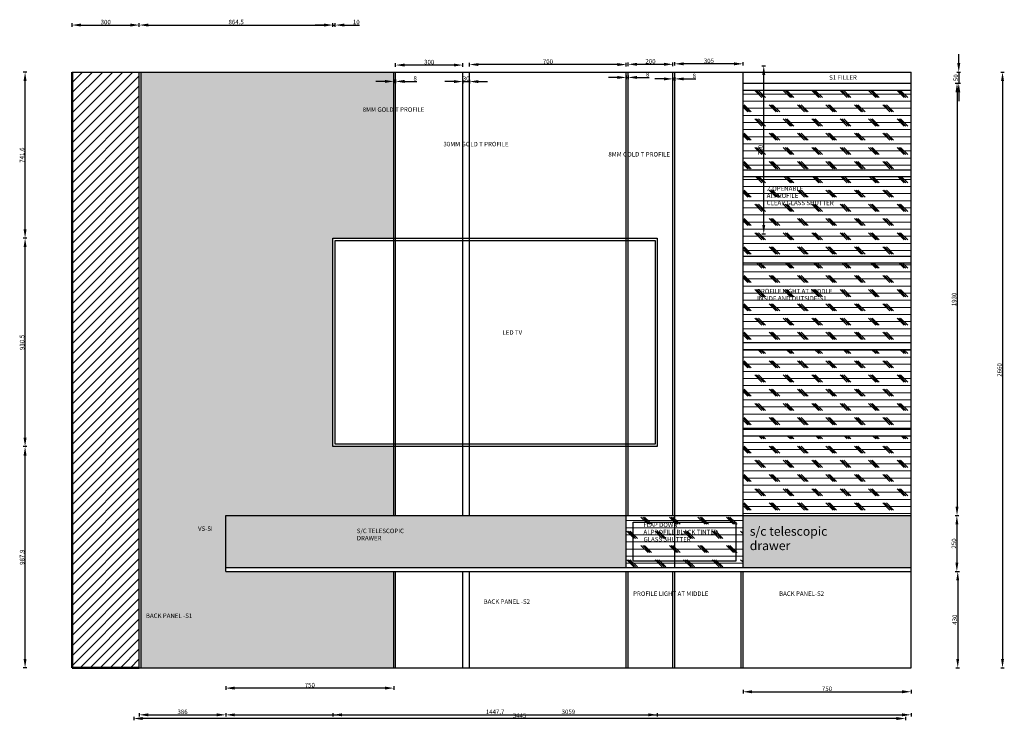
# Model space of a CAD drawing. Units: millimetres. Extents: x -4231 to 8464, y -424 to 4269.
# Tile 2 of 2: x 4069 to 8464, y 1141 to 4269. Entities that reach past the tile are written whole.
import ezdxf

# ---------------------------------------------------------------- set-up
doc = ezdxf.new("R2010")
doc.units = ezdxf.units.MM
for name, color, linetype, lineweight in [('A-ANNO-DIMS', 2, 'Continuous', 18), ('A-ANNO-TEXT', 3, 'Continuous', 18), ('A-EQPM', 6, 'Continuous', 25), ('A-FURN', 30, 'Continuous', 25), ('A-FURN-PATT', 252, 'Continuous', 13), ('A-WALL', 7, 'Continuous', 50), ('A-WALL-PATT', 8, 'Continuous', 13)]:
    doc.layers.add(name, color=color, linetype=linetype, lineweight=lineweight)
doc.styles.get("Standard").update_dxf_attribs({"font": 'arial.ttf', "height": 20})
doc.dimstyles.new('ISO-25', dxfattribs={"dimtxt": 40, "dimasz": 40, "dimexe": 8, "dimexo": 8, "dimtad": 1, "dimdec": 0, "dimtxsty": 'Standard', "dimcen": 2.5, "dimadec": 0, "dimazin": 0, "dimtfac": 1, "dimtdec": 0, "dimtmove": 0, "dimatfit": 3, "dimfxl": 8, "dimfxlon": 1, "dimarcsym": 0})
pattern_1 = [(0, (0, 0), (0, 31.75), []), (135, (15.875, -15.875), (-63.5, -63.5), [44.9013, -44.9013]), (135, (23.81, -15.875), (-63.5, -63.5), [44.9013, -44.9013]), (135, (31.75, -15.875), (-63.5, -63.5), [44.9013, -44.9013])]

# ---------------------------------------------------------------- blocks, each defined once
blk = doc.blocks.new('*D14')
at = {"layer": 'A-ANNO-DIMS', "color": 0, "lineweight": -2, "transparency": 16777216}
for p, q in [((7382.1, 4062.6), (7398.1, 4062.6)), ((7390.1, 3352.6), (7390.1, 4022.6)), ((7382.1, 3312.6), (7398.1, 3312.6))]:
    blk.add_line(p, q, dxfattribs=at)
at = {"layer": 'A-ANNO-DIMS', "color": 0, "transparency": 16777216}
for points in [[(7383.5, 4022.6), (7396.8, 4022.6), (7390.1, 4062.6)], [(7383.5, 3352.6), (7396.8, 3352.6), (7390.1, 3312.6)]]:
    blk.add_solid(points, dxfattribs=at)
at = {"layer": 'Defpoints', "color": 0, "transparency": 16777216}
for p in [(7351.4, 4062.6), (7390.1, 4062.6), (7351.4, 3312.6)]:
    blk.add_point(p, dxfattribs=at)
at = {"layer": 'A-ANNO-DIMS', "color": 0, "transparency": 16777216, "insert": (7379.3, 3687.6), "char_height": 20, "attachment_point": 5, "rotation": 90}
blk.add_mtext('750', dxfattribs=at)
blk = doc.blocks.new('*D15')
at = {"layer": 'A-ANNO-DIMS', "color": 0, "lineweight": -2, "transparency": 16777216}
for p, q in [((6784.7, 4061.8), (6784.7, 4077.8)), ((6824.7, 4069.8), (6944.7, 4069.8)), ((6984.7, 4061.8), (6984.7, 4077.8))]:
    blk.add_line(p, q, dxfattribs=at)
at = {"layer": 'A-ANNO-DIMS', "color": 0, "transparency": 16777216}
for points in [[(6824.7, 4076.5), (6824.7, 4063.2), (6784.7, 4069.8)], [(6944.7, 4076.5), (6944.7, 4063.2), (6984.7, 4069.8)]]:
    blk.add_solid(points, dxfattribs=at)
at = {"layer": 'Defpoints', "color": 0, "transparency": 16777216}
for p in [(6984.7, 4069.8), (6784.7, 4035), (6984.7, 4035)]:
    blk.add_point(p, dxfattribs=at)
at = {"layer": 'A-ANNO-DIMS', "color": 0, "transparency": 16777216, "insert": (6884.7, 4080.7), "char_height": 20, "attachment_point": 5}
blk.add_mtext('200', dxfattribs=at)
blk = doc.blocks.new('*D16')
at = {"layer": 'A-ANNO-DIMS', "color": 0, "lineweight": -2, "transparency": 16777216}
for p, q in [((6992.7, 4063.8), (6992.7, 4079.8)), ((7257.7, 4071.8), (7032.7, 4071.8)), ((7297.7, 4063.8), (7297.7, 4079.8))]:
    blk.add_line(p, q, dxfattribs=at)
at = {"layer": 'A-ANNO-DIMS', "color": 0, "transparency": 16777216}
for points in [[(7032.7, 4078.5), (7032.7, 4065.1), (6992.7, 4071.8)], [(7257.7, 4078.5), (7257.7, 4065.1), (7297.7, 4071.8)]]:
    blk.add_solid(points, dxfattribs=at)
at = {"layer": 'Defpoints', "color": 0, "transparency": 16777216}
for p in [(6992.7, 4071.8), (6992.7, 4035), (7297.7, 4035)]:
    blk.add_point(p, dxfattribs=at)
at = {"layer": 'A-ANNO-DIMS', "color": 0, "transparency": 16777216, "insert": (7145.2, 4082.7), "char_height": 20, "attachment_point": 5}
blk.add_mtext('305', dxfattribs=at)
blk = doc.blocks.new('*D17')
at = {"layer": 'A-ANNO-DIMS', "color": 0, "lineweight": -2, "transparency": 16777216}
for p, q in [((6076.7, 4060.7), (6076.7, 4076.7)), ((6736.7, 4068.7), (6116.7, 4068.7)), ((6776.7, 4060.7), (6776.7, 4076.7))]:
    blk.add_line(p, q, dxfattribs=at)
at = {"layer": 'A-ANNO-DIMS', "color": 0, "transparency": 16777216}
for points in [[(6116.7, 4075.3), (6116.7, 4062), (6076.7, 4068.7)], [(6736.7, 4075.3), (6736.7, 4062), (6776.7, 4068.7)]]:
    blk.add_solid(points, dxfattribs=at)
at = {"layer": 'Defpoints', "color": 0, "transparency": 16777216}
for p in [(6076.7, 4068.7), (6076.7, 4035), (6776.7, 4035)]:
    blk.add_point(p, dxfattribs=at)
at = {"layer": 'A-ANNO-DIMS', "color": 0, "transparency": 16777216, "insert": (6426.7, 4079.5), "char_height": 20, "attachment_point": 5}
blk.add_mtext('700', dxfattribs=at)
blk = doc.blocks.new('*D18')
at = {"layer": 'A-ANNO-DIMS', "color": 0, "lineweight": -2, "transparency": 16777216}
for p, q in [((5746.7, 4058.4), (5746.7, 4074.4)), ((6006.7, 4066.4), (5786.7, 4066.4)), ((6046.7, 4058.4), (6046.7, 4074.4))]:
    blk.add_line(p, q, dxfattribs=at)
at = {"layer": 'A-ANNO-DIMS', "color": 0, "transparency": 16777216}
for points in [[(5786.7, 4073.1), (5786.7, 4059.8), (5746.7, 4066.4)], [(6006.7, 4073.1), (6006.7, 4059.8), (6046.7, 4066.4)]]:
    blk.add_solid(points, dxfattribs=at)
at = {"layer": 'Defpoints', "color": 0, "transparency": 16777216}
for p in [(5746.7, 4066.4), (5746.7, 4035), (6046.7, 4035)]:
    blk.add_point(p, dxfattribs=at)
at = {"layer": 'A-ANNO-DIMS', "color": 0, "transparency": 16777216, "insert": (5896.7, 4077.3), "char_height": 20, "attachment_point": 5}
blk.add_mtext('300', dxfattribs=at)
blk = doc.blocks.new('*D19')
at = {"layer": 'A-ANNO-DIMS', "color": 0, "lineweight": -2, "transparency": 16777216}
for p, q in [((8260.7, 4075), (8260.7, 4115)), ((8252.7, 4035), (8268.7, 4035)), ((8260.7, 4035), (8260.7, 3985)), ((8252.7, 3985), (8268.7, 3985)), ((8260.7, 3945), (8260.7, 3905))]:
    blk.add_line(p, q, dxfattribs=at)
at = {"layer": 'A-ANNO-DIMS', "color": 0, "transparency": 16777216}
for points in [[(8254, 4075), (8267.3, 4075), (8260.7, 4035)], [(8254, 3945), (8267.3, 3945), (8260.7, 3985)]]:
    blk.add_solid(points, dxfattribs=at)
at = {"layer": 'Defpoints', "color": 0, "transparency": 16777216}
for p in [(8047.7, 4035), (8047.7, 3985), (8260.7, 3985)]:
    blk.add_point(p, dxfattribs=at)
at = {"layer": 'A-ANNO-DIMS', "color": 0, "transparency": 16777216, "insert": (8249.8, 4010), "char_height": 20, "attachment_point": 5, "rotation": 90}
blk.add_mtext('50', dxfattribs=at)
blk = doc.blocks.new('*D20')
at = {"layer": 'A-ANNO-DIMS', "color": 0, "lineweight": -2, "transparency": 16777216}
for p, q in [((8245, 3985), (8261, 3985)), ((8253, 3945), (8253, 2095)), ((8245, 2055), (8261, 2055))]:
    blk.add_line(p, q, dxfattribs=at)
at = {"layer": 'A-ANNO-DIMS', "color": 0, "transparency": 16777216}
for points in [[(8246.3, 3945), (8259.6, 3945), (8253, 3985)], [(8246.3, 2095), (8259.6, 2095), (8253, 2055)]]:
    blk.add_solid(points, dxfattribs=at)
at = {"layer": 'Defpoints', "color": 0, "transparency": 16777216}
for p in [(8047.7, 3985), (8047.7, 2055), (8253, 2055)]:
    blk.add_point(p, dxfattribs=at)
at = {"layer": 'A-ANNO-DIMS', "color": 0, "transparency": 16777216, "insert": (8242.1, 3020), "char_height": 20, "attachment_point": 5, "rotation": 90}
blk.add_mtext('1930', dxfattribs=at)
blk = doc.blocks.new('*D21')
at = {"layer": 'A-ANNO-DIMS', "color": 0, "lineweight": -2, "transparency": 16777216}
for p, q in [((8448, 4035), (8464, 4035)), ((8456, 3995), (8456, 1415)), ((8448, 1375), (8464, 1375))]:
    blk.add_line(p, q, dxfattribs=at)
at = {"layer": 'A-ANNO-DIMS', "color": 0, "transparency": 16777216}
for points in [[(8449.4, 3995), (8462.7, 3995), (8456, 4035)], [(8449.4, 1415), (8462.7, 1415), (8456, 1375)]]:
    blk.add_solid(points, dxfattribs=at)
at = {"layer": 'Defpoints', "color": 0, "transparency": 16777216}
for p in [(8047.7, 4035), (8047.7, 1375), (8456, 1375)]:
    blk.add_point(p, dxfattribs=at)
at = {"layer": 'A-ANNO-DIMS', "color": 0, "transparency": 16777216, "insert": (8445.2, 2705), "char_height": 20, "attachment_point": 5, "rotation": 90}
blk.add_mtext('2660', dxfattribs=at)
blk = doc.blocks.new('*D22')
at = {"layer": 'A-ANNO-DIMS', "color": 0, "lineweight": -2, "transparency": 16777216}
for p, q in [((8248.1, 1805), (8264.1, 1805)), ((8256.1, 1765), (8256.1, 1415)), ((8248.1, 1375), (8264.1, 1375))]:
    blk.add_line(p, q, dxfattribs=at)
at = {"layer": 'A-ANNO-DIMS', "color": 0, "transparency": 16777216}
for points in [[(8249.4, 1765), (8262.7, 1765), (8256.1, 1805)], [(8249.4, 1415), (8262.7, 1415), (8256.1, 1375)]]:
    blk.add_solid(points, dxfattribs=at)
at = {"layer": 'Defpoints', "color": 0, "transparency": 16777216}
for p in [(8047.7, 1805), (8047.7, 1375), (8256.1, 1375)]:
    blk.add_point(p, dxfattribs=at)
at = {"layer": 'A-ANNO-DIMS', "color": 0, "transparency": 16777216, "insert": (8245.2, 1590), "char_height": 20, "attachment_point": 5, "rotation": 90}
blk.add_mtext('430', dxfattribs=at)
blk = doc.blocks.new('*D23')
at = {"layer": 'A-ANNO-DIMS', "color": 0, "lineweight": -2, "transparency": 16777216}
for p, q in [((8244.3, 2055), (8260.3, 2055)), ((8252.3, 2015), (8252.3, 1845)), ((8244.3, 1805), (8260.3, 1805))]:
    blk.add_line(p, q, dxfattribs=at)
at = {"layer": 'A-ANNO-DIMS', "color": 0, "transparency": 16777216}
for points in [[(8245.7, 2015), (8259, 2015), (8252.3, 2055)], [(8245.7, 1845), (8259, 1845), (8252.3, 1805)]]:
    blk.add_solid(points, dxfattribs=at)
at = {"layer": 'Defpoints', "color": 0, "transparency": 16777216}
for p in [(8047.7, 2055), (8047.7, 1805), (8252.3, 1805)]:
    blk.add_point(p, dxfattribs=at)
at = {"layer": 'A-ANNO-DIMS', "color": 0, "transparency": 16777216, "insert": (8241.5, 1930), "char_height": 20, "attachment_point": 5, "rotation": 90}
blk.add_mtext('250', dxfattribs=at)
blk = doc.blocks.new('*D24')
at = {"layer": 'A-ANNO-DIMS', "color": 0, "lineweight": -2, "transparency": 16777216}
for p, q in [((7297.7, 1276.1), (7297.7, 1260.1)), ((8047.7, 1276.1), (8047.7, 1260.1)), ((7337.7, 1268.1), (8007.7, 1268.1))]:
    blk.add_line(p, q, dxfattribs=at)
at = {"layer": 'A-ANNO-DIMS', "color": 0, "transparency": 16777216}
for points in [[(7337.7, 1274.8), (7337.7, 1261.4), (7297.7, 1268.1)], [(8007.7, 1274.8), (8007.7, 1261.4), (8047.7, 1268.1)]]:
    blk.add_solid(points, dxfattribs=at)
at = {"layer": 'Defpoints', "color": 0, "transparency": 16777216}
for p in [(7297.7, 1823), (8047.7, 1823), (8047.7, 1268.1)]:
    blk.add_point(p, dxfattribs=at)
at = {"layer": 'A-ANNO-DIMS', "color": 0, "transparency": 16777216, "insert": (7672.7, 1278.9), "char_height": 20, "attachment_point": 5}
blk.add_mtext('750', dxfattribs=at)
blk = doc.blocks.new('*D25')
at = {"layer": 'A-ANNO-DIMS', "color": 0, "lineweight": -2, "transparency": 16777216}
for p, q in [((4988.7, 1292.4), (4988.7, 1276.4)), ((5698.7, 1284.4), (5028.7, 1284.4)), ((5738.7, 1292.4), (5738.7, 1276.4))]:
    blk.add_line(p, q, dxfattribs=at)
at = {"layer": 'A-ANNO-DIMS', "color": 0, "transparency": 16777216}
for points in [[(5028.7, 1291.1), (5028.7, 1277.7), (4988.7, 1284.4)], [(5698.7, 1291.1), (5698.7, 1277.7), (5738.7, 1284.4)]]:
    blk.add_solid(points, dxfattribs=at)
at = {"layer": 'Defpoints', "color": 0, "transparency": 16777216}
for p in [(4988.7, 1375), (5738.7, 1375), (4988.7, 1284.4)]:
    blk.add_point(p, dxfattribs=at)
at = {"layer": 'A-ANNO-DIMS', "color": 0, "transparency": 16777216, "insert": (5363.7, 1295.2), "char_height": 20, "attachment_point": 5}
blk.add_mtext('750', dxfattribs=at)
blk = doc.blocks.new('*D26')
at = {"layer": 'A-ANNO-DIMS', "color": 0, "lineweight": -2, "transparency": 16777216}
for p, q in [((4577.6, 1156.6), (4577.6, 1140.6)), ((7982.6, 1148.6), (4617.6, 1148.6)), ((8022.6, 1156.6), (8022.6, 1140.6))]:
    blk.add_line(p, q, dxfattribs=at)
at = {"layer": 'A-ANNO-DIMS', "color": 0, "transparency": 16777216}
for points in [[(4617.6, 1155.3), (4617.6, 1141.9), (4577.6, 1148.6)], [(7982.6, 1155.3), (7982.6, 1141.9), (8022.6, 1148.6)]]:
    blk.add_solid(points, dxfattribs=at)
at = {"layer": 'Defpoints', "color": 0, "transparency": 16777216}
for p in [(4577.6, 1631.7), (8022.6, 1631.7), (4577.6, 1148.6)]:
    blk.add_point(p, dxfattribs=at)
at = {"layer": 'A-ANNO-DIMS', "color": 0, "transparency": 16777216, "insert": (6300.1, 1159.4), "char_height": 20, "attachment_point": 5}
blk.add_mtext('3445', dxfattribs=at)
blk = doc.blocks.new('*D27')
at = {"layer": 'A-ANNO-DIMS', "color": 0, "lineweight": -2, "transparency": 16777216}
for p, q in [((5738.7, 4001.3), (5738.7, 3985.3)), ((5746.7, 4001.3), (5746.7, 3985.3)), ((5698.7, 3993.3), (5658.7, 3993.3)), ((5738.7, 3993.3), (5746.7, 3993.3)), ((5786.7, 3993.3), (5841.1, 3993.3))]:
    blk.add_line(p, q, dxfattribs=at)
at = {"layer": 'A-ANNO-DIMS', "color": 0, "transparency": 16777216}
for points in [[(5698.7, 4000), (5698.7, 3986.6), (5738.7, 3993.3)], [(5786.7, 4000), (5786.7, 3986.6), (5746.7, 3993.3)]]:
    blk.add_solid(points, dxfattribs=at)
at = {"layer": 'Defpoints', "color": 0, "transparency": 16777216}
for p in [(5738.7, 4035), (5746.7, 4035), (5746.7, 3993.3)]:
    blk.add_point(p, dxfattribs=at)
at = {"layer": 'A-ANNO-DIMS', "color": 0, "transparency": 16777216, "insert": (5833.9, 4004.1), "char_height": 20, "attachment_point": 5}
blk.add_mtext('8', dxfattribs=at)
blk = doc.blocks.new('*D28')
at = {"layer": 'A-ANNO-DIMS', "color": 0, "lineweight": -2, "transparency": 16777216}
for p, q in [((6046.7, 4000.6), (6046.7, 3984.6)), ((6076.7, 4000.6), (6076.7, 3984.6)), ((6006.7, 3992.6), (5966.7, 3992.6)), ((6046.7, 3992.6), (6076.7, 3992.6)), ((6116.7, 3992.6), (6156.7, 3992.6))]:
    blk.add_line(p, q, dxfattribs=at)
at = {"layer": 'A-ANNO-DIMS', "color": 0, "transparency": 16777216}
for points in [[(6006.7, 3999.2), (6006.7, 3985.9), (6046.7, 3992.6)], [(6116.7, 3999.2), (6116.7, 3985.9), (6076.7, 3992.6)]]:
    blk.add_solid(points, dxfattribs=at)
at = {"layer": 'Defpoints', "color": 0, "transparency": 16777216}
for p in [(6046.7, 4035), (6076.7, 4035), (6076.7, 3992.6)]:
    blk.add_point(p, dxfattribs=at)
at = {"layer": 'A-ANNO-DIMS', "color": 0, "transparency": 16777216, "insert": (6061.7, 4003.4), "char_height": 20, "attachment_point": 5}
blk.add_mtext('30', dxfattribs=at)
blk = doc.blocks.new('*D29')
at = {"layer": 'A-ANNO-DIMS', "color": 0, "lineweight": -2, "transparency": 16777216}
for p, q in [((6736.7, 4011.1), (6696.7, 4011.1)), ((6776.7, 4019.1), (6776.7, 4003.1)), ((6776.7, 4011.1), (6784.7, 4011.1)), ((6784.7, 4019.1), (6784.7, 4003.1)), ((6824.7, 4011.1), (6879.1, 4011.1))]:
    blk.add_line(p, q, dxfattribs=at)
at = {"layer": 'A-ANNO-DIMS', "color": 0, "transparency": 16777216}
for points in [[(6736.7, 4017.8), (6736.7, 4004.5), (6776.7, 4011.1)], [(6824.7, 4017.8), (6824.7, 4004.5), (6784.7, 4011.1)]]:
    blk.add_solid(points, dxfattribs=at)
at = {"layer": 'Defpoints', "color": 0, "transparency": 16777216}
for p in [(6776.7, 4035), (6784.7, 4035), (6784.7, 4011.1)]:
    blk.add_point(p, dxfattribs=at)
at = {"layer": 'A-ANNO-DIMS', "color": 0, "transparency": 16777216, "insert": (6871.9, 4022), "char_height": 20, "attachment_point": 5}
blk.add_mtext('8', dxfattribs=at)
blk = doc.blocks.new('*D30')
at = {"layer": 'A-ANNO-DIMS', "color": 0, "lineweight": -2, "transparency": 16777216}
for p, q in [((6944.7, 4004.6), (6904.7, 4004.6)), ((6984.7, 4012.6), (6984.7, 3996.6)), ((6984.7, 4004.6), (6992.7, 4004.6)), ((6992.7, 4012.6), (6992.7, 3996.6)), ((7032.7, 4004.6), (7087.1, 4004.6))]:
    blk.add_line(p, q, dxfattribs=at)
at = {"layer": 'A-ANNO-DIMS', "color": 0, "transparency": 16777216}
for points in [[(6944.7, 4011.2), (6944.7, 3997.9), (6984.7, 4004.6)], [(7032.7, 4011.2), (7032.7, 3997.9), (6992.7, 4004.6)]]:
    blk.add_solid(points, dxfattribs=at)
at = {"layer": 'Defpoints', "color": 0, "transparency": 16777216}
for p in [(6984.7, 4035), (6992.7, 4035), (6992.7, 4004.6)]:
    blk.add_point(p, dxfattribs=at)
at = {"layer": 'A-ANNO-DIMS', "color": 0, "transparency": 16777216, "insert": (7079.9, 4015.4), "char_height": 20, "attachment_point": 5}
blk.add_mtext('8', dxfattribs=at)
blk = doc.blocks.new('*D34')
at = {"layer": 'A-ANNO-DIMS', "color": 0, "lineweight": -2, "transparency": 16777216}
for p, q in [((4302.7, 4237), (4302.7, 4253)), ((4342.7, 4245), (4562.7, 4245)), ((4602.7, 4237), (4602.7, 4253))]:
    blk.add_line(p, q, dxfattribs=at)
at = {"layer": 'A-ANNO-DIMS', "color": 0, "transparency": 16777216}
for points in [[(4342.7, 4251.7), (4342.7, 4238.4), (4302.7, 4245)], [(4562.7, 4251.7), (4562.7, 4238.4), (4602.7, 4245)]]:
    blk.add_solid(points, dxfattribs=at)
at = {"layer": 'Defpoints', "color": 0, "transparency": 16777216}
for p in [(4602.7, 4245), (4302.7, 4035), (4602.7, 4035)]:
    blk.add_point(p, dxfattribs=at)
at = {"layer": 'A-ANNO-DIMS', "color": 0, "transparency": 16777216, "insert": (4452.7, 4255.9), "char_height": 20, "attachment_point": 5}
blk.add_mtext('300', dxfattribs=at)
blk = doc.blocks.new('*D35')
at = {"layer": 'A-ANNO-DIMS', "color": 0, "lineweight": -2, "transparency": 16777216}
for p, q in [((4602.7, 4237), (4602.7, 4253)), ((4642.7, 4245), (5427.2, 4245)), ((5467.2, 4237), (5467.2, 4253))]:
    blk.add_line(p, q, dxfattribs=at)
at = {"layer": 'A-ANNO-DIMS', "color": 0, "transparency": 16777216}
for points in [[(4642.7, 4251.7), (4642.7, 4238.4), (4602.7, 4245)], [(5427.2, 4251.7), (5427.2, 4238.4), (5467.2, 4245)]]:
    blk.add_solid(points, dxfattribs=at)
at = {"layer": 'Defpoints', "color": 0, "transparency": 16777216}
for p in [(5467.2, 4245), (4602.7, 4035), (5467.2, 3293.4)]:
    blk.add_point(p, dxfattribs=at)
at = {"layer": 'A-ANNO-DIMS', "color": 0, "transparency": 16777216, "insert": (5034.9, 4255.9), "char_height": 20, "attachment_point": 5}
blk.add_mtext('864.5', dxfattribs=at)
blk = doc.blocks.new('*D36')
at = {"layer": 'A-ANNO-DIMS', "color": 0, "lineweight": -2, "transparency": 16777216}
for p, q in [((5427.2, 4245), (5387.2, 4245)), ((5467.2, 4237), (5467.2, 4253)), ((5467.2, 4245), (5477.2, 4245)), ((5477.2, 4237), (5477.2, 4253)), ((5517.2, 4245), (5585.1, 4245))]:
    blk.add_line(p, q, dxfattribs=at)
at = {"layer": 'A-ANNO-DIMS', "color": 0, "transparency": 16777216}
for points in [[(5427.2, 4251.7), (5427.2, 4238.4), (5467.2, 4245)], [(5517.2, 4251.7), (5517.2, 4238.4), (5477.2, 4245)]]:
    blk.add_solid(points, dxfattribs=at)
at = {"layer": 'Defpoints', "color": 0, "transparency": 16777216}
for p in [(5477.2, 4245), (5467.2, 3293.4), (5477.2, 3283.4)]:
    blk.add_point(p, dxfattribs=at)
at = {"layer": 'A-ANNO-DIMS', "color": 0, "transparency": 16777216, "insert": (5571.2, 4255.9), "char_height": 20, "attachment_point": 5}
blk.add_mtext('10', dxfattribs=at)
blk = doc.blocks.new('*D37')
at = {"layer": 'A-ANNO-DIMS', "color": 0, "lineweight": -2, "transparency": 16777216}
for p, q in [((4602.7, 1173), (4602.7, 1157)), ((4642.7, 1165), (4948.7, 1165)), ((4988.7, 1173), (4988.7, 1157))]:
    blk.add_line(p, q, dxfattribs=at)
at = {"layer": 'A-ANNO-DIMS', "color": 0, "transparency": 16777216}
for points in [[(4642.7, 1171.7), (4642.7, 1158.4), (4602.7, 1165)], [(4948.7, 1171.7), (4948.7, 1158.4), (4988.7, 1165)]]:
    blk.add_solid(points, dxfattribs=at)
at = {"layer": 'Defpoints', "color": 0, "transparency": 16777216}
for p in [(4988.7, 1805), (4602.7, 1375), (4988.7, 1165)]:
    blk.add_point(p, dxfattribs=at)
at = {"layer": 'A-ANNO-DIMS', "color": 0, "transparency": 16777216, "insert": (4795.7, 1175.9), "char_height": 20, "attachment_point": 5}
blk.add_mtext('386', dxfattribs=at)
blk = doc.blocks.new('*D38')
at = {"layer": 'A-ANNO-DIMS', "color": 0, "lineweight": -2, "transparency": 16777216}
for p, q in [((4988.7, 1173), (4988.7, 1157)), ((5028.7, 1165), (8007.7, 1165)), ((8047.7, 1173), (8047.7, 1157))]:
    blk.add_line(p, q, dxfattribs=at)
at = {"layer": 'A-ANNO-DIMS', "color": 0, "transparency": 16777216}
for points in [[(5028.7, 1171.7), (5028.7, 1158.4), (4988.7, 1165)], [(8007.7, 1171.7), (8007.7, 1158.4), (8047.7, 1165)]]:
    blk.add_solid(points, dxfattribs=at)
at = {"layer": 'Defpoints', "color": 0, "transparency": 16777216}
for p in [(4988.7, 1805), (8047.7, 1375), (8047.7, 1165)]:
    blk.add_point(p, dxfattribs=at)
at = {"layer": 'A-ANNO-DIMS', "color": 0, "transparency": 16777216, "insert": (6518.2, 1175.9), "char_height": 20, "attachment_point": 5}
blk.add_mtext('3059', dxfattribs=at)
blk = doc.blocks.new('*D39')
at = {"layer": 'A-ANNO-DIMS', "color": 0, "lineweight": -2, "transparency": 16777216}
for p, q in [((5467.2, 1173), (5467.2, 1157)), ((5507.2, 1165), (6874.9, 1165)), ((6914.9, 1173), (6914.9, 1157))]:
    blk.add_line(p, q, dxfattribs=at)
at = {"layer": 'A-ANNO-DIMS', "color": 0, "transparency": 16777216}
for points in [[(5507.2, 1171.7), (5507.2, 1158.4), (5467.2, 1165)], [(6874.9, 1171.7), (6874.9, 1158.4), (6914.9, 1165)]]:
    blk.add_solid(points, dxfattribs=at)
at = {"layer": 'Defpoints', "color": 0, "transparency": 16777216}
for p in [(5467.2, 2362.9), (6914.9, 2362.9), (6914.9, 1165)]:
    blk.add_point(p, dxfattribs=at)
at = {"layer": 'A-ANNO-DIMS', "color": 0, "transparency": 16777216, "insert": (6191, 1175.7), "char_height": 20, "attachment_point": 5}
blk.add_mtext('1447.7', dxfattribs=at)
blk = doc.blocks.new('*D40')
at = {"layer": 'A-ANNO-DIMS', "color": 0, "lineweight": -2, "transparency": 16777216}
for p, q in [((4100.7, 2362.9), (4084.7, 2362.9)), ((4092.7, 1415), (4092.7, 2322.9)), ((4100.7, 1375), (4084.7, 1375))]:
    blk.add_line(p, q, dxfattribs=at)
at = {"layer": 'A-ANNO-DIMS', "color": 0, "transparency": 16777216}
for points in [[(4086, 2322.9), (4099.3, 2322.9), (4092.7, 2362.9)], [(4086, 1415), (4099.3, 1415), (4092.7, 1375)]]:
    blk.add_solid(points, dxfattribs=at)
at = {"layer": 'Defpoints', "color": 0, "transparency": 16777216}
for p in [(4092.7, 2362.9), (5467.2, 2362.9), (4302.7, 1375)]:
    blk.add_point(p, dxfattribs=at)
at = {"layer": 'A-ANNO-DIMS', "color": 0, "transparency": 16777216, "insert": (4081.8, 1869), "char_height": 20, "attachment_point": 5, "rotation": 90}
blk.add_mtext('987.9', dxfattribs=at)
blk = doc.blocks.new('*D41')
at = {"layer": 'A-ANNO-DIMS', "color": 0, "lineweight": -2, "transparency": 16777216}
for p, q in [((4100.7, 3293.4), (4084.7, 3293.4)), ((4092.7, 2402.9), (4092.7, 3253.4)), ((4100.7, 2362.9), (4084.7, 2362.9))]:
    blk.add_line(p, q, dxfattribs=at)
at = {"layer": 'A-ANNO-DIMS', "color": 0, "transparency": 16777216}
for points in [[(4086, 3253.4), (4099.3, 3253.4), (4092.7, 3293.4)], [(4086, 2402.9), (4099.3, 2402.9), (4092.7, 2362.9)]]:
    blk.add_solid(points, dxfattribs=at)
at = {"layer": 'Defpoints', "color": 0, "transparency": 16777216}
for p in [(4092.7, 3293.4), (5467.2, 3293.4), (5467.2, 2362.9)]:
    blk.add_point(p, dxfattribs=at)
at = {"layer": 'A-ANNO-DIMS', "color": 0, "transparency": 16777216, "insert": (4081.8, 2828.1), "char_height": 20, "attachment_point": 5, "rotation": 90}
blk.add_mtext('930.5', dxfattribs=at)
blk = doc.blocks.new('*D42')
at = {"layer": 'A-ANNO-DIMS', "color": 0, "lineweight": -2, "transparency": 16777216}
for p, q in [((4100.7, 4035), (4084.7, 4035)), ((4092.7, 3333.4), (4092.7, 3995)), ((4100.7, 3293.4), (4084.7, 3293.4))]:
    blk.add_line(p, q, dxfattribs=at)
at = {"layer": 'A-ANNO-DIMS', "color": 0, "transparency": 16777216}
for points in [[(4086, 3995), (4099.3, 3995), (4092.7, 4035)], [(4086, 3333.4), (4099.3, 3333.4), (4092.7, 3293.4)]]:
    blk.add_solid(points, dxfattribs=at)
at = {"layer": 'Defpoints', "color": 0, "transparency": 16777216}
for p in [(4092.7, 4035), (4302.7, 4035), (5467.2, 3293.4)]:
    blk.add_point(p, dxfattribs=at)
at = {"layer": 'A-ANNO-DIMS', "color": 0, "transparency": 16777216, "insert": (4081.8, 3664.2), "char_height": 20, "attachment_point": 5, "rotation": 90}
blk.add_mtext('741.6', dxfattribs=at)

msp = doc.modelspace()

# ---------------------------------------------------------------- hatches: boundary and pattern name
at = {"layer": 'A-FURN-PATT'}
h = msp.add_hatch(dxfattribs=at)
h.set_pattern_fill('GOST_WOOD', color=256, scale=10)
h.paths.add_polyline_path([(5738.65, 4035.02), (4610.65, 4035.02), (4610.65, 1375.02), (5738.65, 1375.02), (5738.65, 1805.02), (4988.65, 1805.02), (4988.65, 2055.02), (5738.65, 2055.02), (5738.65, 2362.91), (5467.19, 2362.91), (5467.19, 3293.39), (5738.65, 3293.39)])
h.paths.add_polyline_path([(6776.65, 2055.02), (4988.65, 2055.02), (4988.65, 1823.02), (6776.65, 1823.02)])
h.paths.add_polyline_path([(8047.65, 2055.02), (7297.65, 2055.02), (7297.65, 1823.02), (8047.65, 1823.02)])
h.paths.add_polyline_path([(4626.95, 1591.95), (4864, 1591.95), (4864, 1622.97), (4626.95, 1622.97)], flags=24)
h.paths.add_polyline_path([(4859.72, 1980.87), (4943.03, 1980.87), (4943.03, 2011.9), (4859.72, 2011.9)], flags=24)
h.paths.add_polyline_path([(5568.61, 1939.16), (5702.79, 1939.16), (5702.79, 1969.16), (5568.61, 1969.16)], flags=24)
h.paths.add_polyline_path([(5568.44, 1970.77), (5810.12, 1970.77), (5810.12, 2001.81), (5568.44, 2001.81)], flags=24)
h.paths.add_polyline_path([(7317.55, 1889.74), (7509.45, 1889.74), (7509.45, 1950.72), (7317.55, 1950.72)], flags=24)
h.paths.add_polyline_path([(7314.77, 1940.76), (7691.61, 1940.76), (7691.61, 2018.44), (7314.77, 2018.44)], flags=24)
h = msp.add_hatch(dxfattribs=at)
h.set_pattern_fill('CORK', color=256, scale=10)
h.set_pattern_definition(pattern_1)
h.paths.add_polyline_path([(8047.65, 3955.02), (7297.65, 3955.02), (7297.65, 3599.02), (8047.65, 3599.02)])
h.paths.add_polyline_path([(8047.65, 3569.02), (7297.65, 3569.02), (7297.65, 3213.02), (8047.65, 3213.02)])
h.paths.add_polyline_path([(8047.65, 3183.02), (7297.65, 3183.02), (7297.65, 2827.02), (8047.65, 2827.02)])
h.paths.add_polyline_path([(8047.65, 2797.02), (7297.65, 2797.02), (7297.65, 2441.02), (8047.65, 2441.02)])
h.paths.add_polyline_path([(8047.65, 2411.02), (7297.65, 2411.02), (7297.65, 2055.02), (8047.65, 2055.02)])
h = msp.add_hatch(dxfattribs=at)
h.set_pattern_fill('CORK', color=256, scale=10)
h.set_pattern_definition(pattern_1)
h.paths.add_polyline_path([(7267.65, 2025.02), (6992.65, 2025.02), (6806.65, 2025.02), (6806.65, 1853.02), (7267.65, 1853.02)], flags=0)
h.paths.add_polyline_path([(7297.65, 2055.02), (6992.65, 2055.02), (6776.65, 2055.02), (6776.65, 1823.02), (7297.65, 1823.02)])
h.paths.add_polyline_path([(7267.65, 1853.02), (6806.65, 1853.02), (6806.65, 2025.02), (6992.65, 2025.02), (7267.65, 2025.02)], flags=16)
h = msp.add_hatch(dxfattribs=at)
h.set_pattern_fill('CORK', color=256, scale=10)
h.set_pattern_definition(pattern_1)
h.paths.add_polyline_path([(7267.65, 2025.02), (6992.65, 2025.02), (6806.65, 2025.02), (6806.65, 1853.02), (7267.65, 1853.02)])
at = {"layer": 'A-WALL-PATT'}
h = msp.add_hatch(dxfattribs=at)
h.set_pattern_fill('ANSI31', color=256, scale=10)
h.paths.add_polyline_path([(4602.65, 4035.02), (4302.65, 4035.02), (4302.65, 1375.02), (4602.65, 1375.02)])

# ---------------------------------------------------------------- linework, layer by layer
at = {"layer": 'A-EQPM'}
for points in [[(5467.19, 3293.39), (6914.85, 3293.39), (6914.85, 2362.91), (5467.19, 2362.91)], [(5477.19, 3283.39), (6904.85, 3283.39), (6904.85, 2372.91), (5477.19, 2372.91)]]:
    msp.add_lwpolyline(points, close=True, dxfattribs=at)
at = {"layer": 'A-FURN'}
for p, q in [((4302.65, 4035.02), (8047.65, 4035.02)), ((4602.65, 1375.02), (4602.65, 4035.02)), ((4610.65, 1375.02), (4610.65, 4035.02)), ((5738.65, 2055.02), (5738.65, 4035.02)), ((5746.65, 2055.02), (5746.65, 4035.02)), ((6046.65, 2055.02), (6046.65, 4035.02)), ((6076.65, 2055.02), (6076.65, 4035.02)), ((6776.65, 1823.02), (6776.65, 4035.02)), ((6784.65, 2055.02), (6784.65, 4035.02)), ((6984.65, 2055.02), (6984.65, 4035.02)), ((6992.65, 2055.02), (6992.65, 4035.02)), ((6992.65, 1823.02), (6992.65, 4035.02)), ((6992.65, 1823.02), (6992.65, 4035.02)), ((6992.65, 1823.02), (6992.65, 4035.02)), ((7297.65, 1823.02), (7297.65, 4035.02)), ((8047.65, 1375.02), (8047.65, 4035.02)), ((7297.65, 3985.02), (8047.65, 3985.02)), ((7297.65, 3955.02), (8047.65, 3955.02)), ((7297.65, 3599.02), (8047.65, 3599.02)), ((7297.65, 3569.02), (8047.65, 3569.02)), ((7297.65, 3213.02), (8047.65, 3213.02)), ((7297.65, 3183.02), (8047.65, 3183.02)), ((7297.65, 2827.02), (8047.65, 2827.02)), ((7297.65, 2797.02), (8047.65, 2797.02)), ((7297.65, 2441.02), (8047.65, 2441.02)), ((7297.65, 2411.02), (8047.65, 2411.02)), ((4988.65, 2055.02), (6992.65, 2055.02)), ((4988.65, 1805.02), (4988.65, 2055.02)), ((6806.65, 2025.02), (6992.65, 2025.02)), ((6806.65, 1853.02), (6806.65, 2025.02)), ((6992.65, 2055.02), (8047.65, 2055.02)), ((6992.65, 2025.02), (7267.65, 2025.02)), ((7267.65, 1853.02), (7267.65, 2025.02)), ((6806.65, 1853.02), (7267.65, 1853.02)), ((4988.65, 1823.02), (8047.65, 1823.02)), ((4988.65, 1805.02), (8047.65, 1805.02)), ((5738.65, 1375.02), (5738.65, 1805.02)), ((5746.65, 1375.02), (5746.65, 1805.02)), ((6046.65, 1375.02), (6046.65, 1805.02)), ((6076.65, 1375.02), (6076.65, 1805.02)), ((6776.65, 1375.02), (6776.65, 1805.02)), ((6784.65, 1375.02), (6784.65, 1805.02)), ((6984.65, 1375.02), (6984.65, 1805.02)), ((6992.65, 1375.02), (6992.65, 1805.02)), ((7289.65, 1375.02), (7289.65, 1805.02)), ((7297.65, 1375.02), (7297.65, 1805.02)), ((4602.65, 1375.02), (8047.65, 1375.02))]:
    msp.add_line(p, q, dxfattribs=at)
at = {"layer": 'A-WALL'}
for p, q in [((4302.65, 1375.02), (4302.65, 4035.02)), ((4602.65, 1375.02), (4302.65, 1375.02))]:
    msp.add_line(p, q, dxfattribs=at)

# ---------------------------------------------------------------- texts
at = {"layer": 'A-ANNO-TEXT'}
for s, height, p in [('S1 FILLER', 20, (7682.18, 4000.52)), ('8MM GOLD T PROFILE', 20, (5600.02, 3857.57)), ('30MM GOLD T PROFILE', 20, (5960.27, 3703.56)), ('8MM GOLD T PROFILE', 20, (6696.51, 3657.91)), ('2-OPENABLE', 20, (7403.33, 3505.02)), ('AI.PROFILE', 20, (7403.33, 3472.9)), ('CLEAR GLASS SHUTTER', 20, (7403.33, 3440.77)), ('PROFILE LIGHT AT MIDDLE', 20, (7360.25, 3047.11)), ('INSIDE AND OUTSIDE-S1', 20, (7360.25, 3014.98)), ('LED TV', 20, (6223.87, 2862.49)), ('FLAP DOWN', 20, (6853.39, 2003.25)), ('VS-SI', 20, (4864.89, 1986.39)), ('S/C TELESCOPIC', 20, (5573.61, 1976.28)), ('AI.PROFILE BLACK TINTED', 20, (6853.39, 1971.12)), ('s/c telescopic ', 40, (7327.72, 1964.81)), ('DRAWER', 20, (5573.61, 1944.16)), ('GLASS SHUTTER', 20, (6853.39, 1938.99)), ('drawer', 40, (7327.72, 1900.56)), ('PROFILE LIGHT AT MIDDLE  ', 20, (6806.87, 1695.92)), ('BACK PANEL-S2', 20, (7458.48, 1696.22)), ('BACK PANEL -S2', 20, (6139.81, 1660.57)), ('BACK PANEL -S1', 20, (4632.12, 1597.46))]:
    msp.add_text(s, height=height, dxfattribs=at).set_placement(p)

# ---------------------------------------------------------------- dimensions: what is measured, and where the dimension line sits
at = {"layer": 'A-ANNO-DIMS'}
for base, p1, p2, override, picture, middle in [((4602.65, 4245.02), (4302.65, 4035.02), (4602.65, 4035.02), {"dimdec": 0, "dimlfac": 1, "dimrnd": 0, "dimzin": 0, "dimdsep": 46, "dimlunit": 2}, '*D34', (4452.65, 4255.86)), ((5467.19, 4245.02), (4602.65, 4035.02), (5467.19, 3293.39), {"dimdec": 1, "dimlfac": 1, "dimrnd": 0, "dimzin": 0, "dimdsep": 46, "dimlunit": 2}, '*D35', (5034.92, 4255.85)), ((5477.19, 4245.02), (5467.19, 3293.39), (5477.19, 3283.39), {"dimdec": 0, "dimlfac": 1, "dimrnd": 0, "dimzin": 0, "dimdsep": 46, "dimlunit": 2}, '*D36', (5571.16, 4255.85)), ((5746.65, 4066.44), (6046.65, 4035.02), (5746.65, 4035.02), {"dimclrd": 0, "dimclre": 0, "dimclrt": 0}, '*D18', (5896.65, 4077.28)), ((6076.65, 4068.65), (6776.65, 4035.02), (6076.65, 4035.02), {"dimclrd": 0, "dimclre": 0, "dimclrt": 0}, '*D17', (6426.65, 4079.49)), ((6984.65, 4069.85), (6784.65, 4035.02), (6984.65, 4035.02), {"dimclrd": 0, "dimclre": 0, "dimclrt": 0}, '*D15', (6884.65, 4080.69)), ((6992.65, 4071.81), (7297.65, 4035.02), (6992.65, 4035.02), {"dimclrd": 0, "dimclre": 0, "dimclrt": 0}, '*D16', (7145.15, 4082.65)), ((5746.65, 3993.31), (5738.65, 4035.02), (5746.65, 4035.02), {"dimclrd": 0, "dimclre": 0, "dimclrt": 0}, '*D27', (5833.87, 4004.15)), ((6076.65, 3992.57), (6046.65, 4035.02), (6076.65, 4035.02), {"dimclrd": 0, "dimclre": 0, "dimclrt": 0}, '*D28', (6061.65, 4003.42)), ((6784.65, 4011.14), (6776.65, 4035.02), (6784.65, 4035.02), {"dimclrd": 0, "dimclre": 0, "dimclrt": 0}, '*D29', (6871.87, 4021.97)), ((6992.65, 4004.56), (6984.65, 4035.02), (6992.65, 4035.02), {"dimclrd": 0, "dimclre": 0, "dimclrt": 0}, '*D30', (7079.87, 4015.4)), ((6914.85, 1165.02), (5467.19, 2362.91), (6914.85, 2362.91), {"dimdec": 1, "dimlfac": 1, "dimrnd": 0, "dimzin": 0, "dimdsep": 46, "dimlunit": 2}, '*D39', (6191.02, 1175.68)), ((4988.65, 1165.02), (4602.65, 1375.02), (4988.65, 1805.02), {"dimdec": 0, "dimlfac": 1, "dimrnd": 0, "dimzin": 0, "dimdsep": 46, "dimlunit": 2}, '*D37', (4795.65, 1175.86)), ((8047.65, 1165.02), (4988.65, 1805.02), (8047.65, 1375.02), {"dimdec": 0, "dimlfac": 1, "dimrnd": 0, "dimzin": 0, "dimdsep": 46, "dimlunit": 2}, '*D38', (6518.15, 1175.86)), ((8047.65, 1268.08), (7297.65, 1823.02), (8047.65, 1823.02), {"dimclrd": 0, "dimclre": 0, "dimclrt": 0}, '*D24', (7672.65, 1278.92)), ((4577.6, 1148.6), (8022.6, 1631.65), (4577.6, 1631.65), {"dimclrd": 0, "dimclre": 0, "dimclrt": 0}, '*D26', (6300.1, 1159.44)), ((4988.65, 1284.39), (5738.65, 1375.02), (4988.65, 1375.02), {"dimclrd": 0, "dimclre": 0, "dimclrt": 0}, '*D25', (5363.65, 1295.23))]:
    dim = msp.add_linear_dim(base=base, p1=p1, p2=p2, dimstyle='ISO-25', override=override, dxfattribs=at)
    dim.commit()
    dim.dimension.update_dxf_attribs({"geometry": picture, "text_midpoint": middle})
for base, p1, p2, angle, override, picture, middle in [((8260.65, 3985.02), (8047.65, 4035.02), (8047.65, 3985.02), 90, {"dimclrd": 0, "dimclre": 0, "dimclrt": 0}, '*D19', (8249.81, 4010.02)), ((7390.14, 4062.63), (7351.43, 3312.63), (7351.43, 4062.63), 270, {"dimclrd": 0, "dimclre": 0, "dimclrt": 0}, '*D14', (7379.3, 3687.63)), ((4092.65, 4035.02), (5467.19, 3293.39), (4302.65, 4035.02), 90, {"dimdec": 1, "dimlfac": 1, "dimrnd": 0, "dimzin": 0, "dimdsep": 46, "dimlunit": 2}, '*D42', (4081.82, 3664.21)), ((8456.03, 1375.02), (8047.65, 4035.02), (8047.65, 1375.02), 90, {"dimclrd": 0, "dimclre": 0, "dimclrt": 0}, '*D21', (8445.19, 2705.02)), ((8252.96, 2055.02), (8047.65, 3985.02), (8047.65, 2055.02), 90, {"dimclrd": 0, "dimclre": 0, "dimclrt": 0}, '*D20', (8242.11, 3020.02)), ((4092.65, 3293.39), (5467.19, 2362.91), (5467.19, 3293.39), 90, {"dimdec": 1, "dimlfac": 1, "dimrnd": 0, "dimzin": 0, "dimdsep": 46, "dimlunit": 2}, '*D41', (4081.81, 2828.15)), ((4092.65, 2362.91), (4302.65, 1375.02), (5467.19, 2362.91), 90, {"dimdec": 1, "dimlfac": 1, "dimrnd": 0, "dimzin": 0, "dimdsep": 46, "dimlunit": 2}, '*D40', (4081.82, 1868.96)), ((8252.33, 1805.02), (8047.65, 2055.02), (8047.65, 1805.02), 90, {"dimclrd": 0, "dimclre": 0, "dimclrt": 0}, '*D23', (8241.49, 1930.02)), ((8256.08, 1375.02), (8047.65, 1805.02), (8047.65, 1375.02), 90, {"dimclrd": 0, "dimclre": 0, "dimclrt": 0}, '*D22', (8245.24, 1590.02))]:
    dim = msp.add_linear_dim(base=base, p1=p1, p2=p2, angle=angle, dimstyle='ISO-25', override=override, dxfattribs=at)
    dim.commit()
    dim.dimension.update_dxf_attribs({"geometry": picture, "text_midpoint": middle})

doc.saveas('drawing.dxf')
